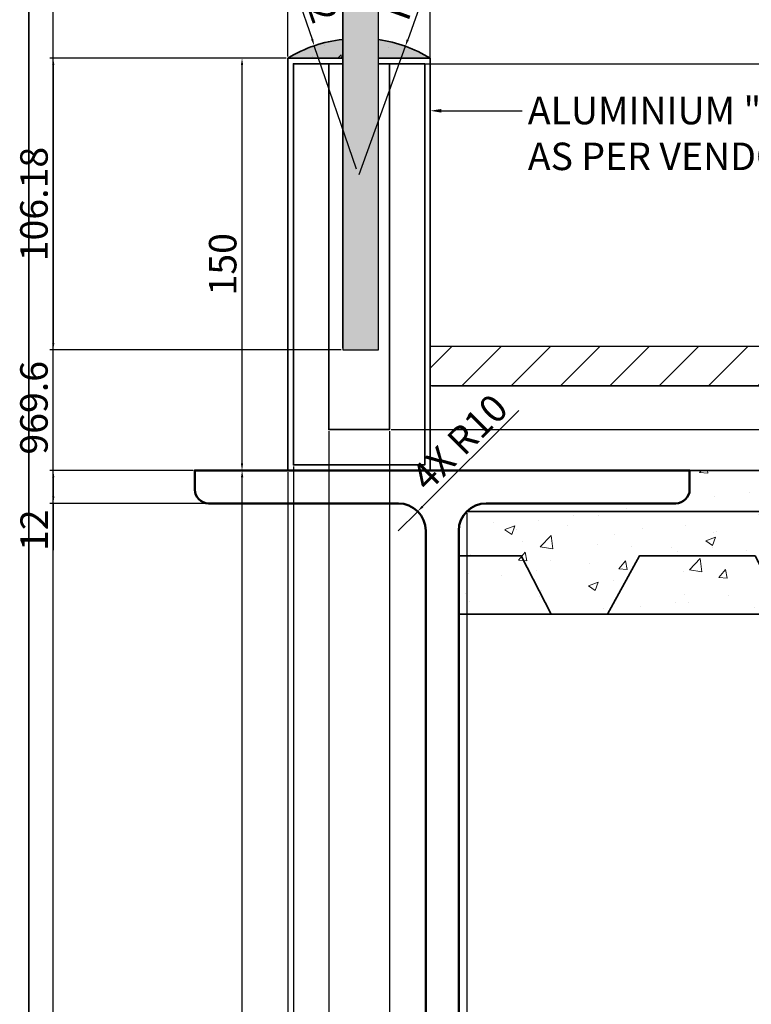
# Model space of a CAD drawing. Units: millimetres. Extents: x 1791 to 2420, y 1225 to 2361.
# Tile 2 of 4: x 1791 to 2057, y 1583 to 1941. Entities that reach past the tile are written whole.
import ezdxf
from ezdxf import colors
from ezdxf.entities.mleader import LeaderData, LeaderLine
from ezdxf.math import Vec2, Vec3

# ---------------------------------------------------------------- set-up
doc = ezdxf.new("R2010")
doc.units = ezdxf.units.MM
for name, color, linetype, lineweight in [('A-ANNO-DIMS', 2, 'Continuous', 18), ('A-ANNO-TEXT', 7, 'Continuous', 18), ('A-ANNO-TTLB', 7, 'Continuous', 35), ('A-DETL-PATT', 8, 'Continuous', 13), ('A-FLOR', 30, 'Continuous', 25), ('A-GLAZ', 5, 'Continuous', 25), ('A-RAIL', 4, 'Continuous', 35), ('S-BEAM', 1, 'Continuous', 50), ('S-DECK', 3, 'Continuous', 35)]:
    doc.layers.add(name, color=color, linetype=linetype, lineweight=lineweight)
doc.styles.get("Standard").update_dxf_attribs({"font": 'arial.ttf'})
doc.dimstyles.new('ISO-25', dxfattribs={"dimtxt": 10, "dimasz": 2.5, "dimexe": 1.25, "dimexo": 0.625, "dimtad": 1, "dimdec": 1, "dimtxsty": 'Standard', "dimcen": 2.5, "dimadec": 0, "dimazin": 0, "dimtfac": 1, "dimtdec": 1, "dimtmove": 0, "dimatfit": 3, "dimfxl": 1, "dimarcsym": 0})

# ---------------------------------------------------------------- blocks, each defined once
blk = doc.blocks.new('*D3')
at = {"layer": 'A-ANNO-DIMS', "color": 0, "lineweight": -2, "transparency": 16777216}
for p, q in [((1860.7, 1777.42), (1873.17, 1777.42)), ((1871.92, 1317.92), (1871.92, 1774.92)), ((1860.7, 1315.42), (1873.17, 1315.42))]:
    blk.add_line(p, q, dxfattribs=at)
at = {"layer": 'A-ANNO-DIMS', "color": 0, "transparency": 16777216}
for points in [[(1871.5, 1774.92), (1872.34, 1774.92), (1871.92, 1777.42)], [(1871.5, 1317.92), (1872.34, 1317.92), (1871.92, 1315.42)]]:
    blk.add_solid(points, dxfattribs=at)
at = {"layer": 'Defpoints', "color": 0, "transparency": 16777216}
for p in [(1860.08, 1777.42), (1871.92, 1777.42), (1860.08, 1315.42)]:
    blk.add_point(p, dxfattribs=at)
at = {"layer": 'A-ANNO-DIMS', "color": 0, "transparency": 16777216, "insert": (1866.19, 1546.42), "char_height": 10, "attachment_point": 5, "rotation": 90}
blk.add_mtext('462', dxfattribs=at)
blk = doc.blocks.new('*D4')
at = {"layer": 'A-ANNO-DIMS', "color": 0, "lineweight": -2, "transparency": 16777216}
for p, q in [((1887.99, 1927.42), (1870.65, 1927.42)), ((1871.9, 1779.92), (1871.9, 1924.92)), ((1887.99, 1777.42), (1870.65, 1777.42))]:
    blk.add_line(p, q, dxfattribs=at)
at = {"layer": 'A-ANNO-DIMS', "color": 0, "transparency": 16777216}
for points in [[(1871.48, 1924.92), (1872.31, 1924.92), (1871.9, 1927.42)], [(1871.48, 1779.92), (1872.31, 1779.92), (1871.9, 1777.42)]]:
    blk.add_solid(points, dxfattribs=at)
at = {"layer": 'Defpoints', "color": 0, "transparency": 16777216}
for p in [(1871.9, 1927.42), (1888.61, 1927.42), (1888.61, 1777.42)]:
    blk.add_point(p, dxfattribs=at)
at = {"layer": 'A-ANNO-DIMS', "color": 0, "transparency": 16777216, "insert": (1866.16, 1852.42), "char_height": 10, "attachment_point": 5, "rotation": 90}
blk.add_mtext('150', dxfattribs=at)
blk = doc.blocks.new('*D11')
at = {"layer": 'A-ANNO-DIMS', "color": 0, "lineweight": -2, "transparency": 16777216}
for p, q in [((1894.37, 2284.98), (1801.98, 2284.98)), ((1803.23, 1317.92), (1803.23, 2282.48)), ((1854.1, 1315.42), (1801.98, 1315.42))]:
    blk.add_line(p, q, dxfattribs=at)
at = {"layer": 'A-ANNO-DIMS', "color": 0, "transparency": 16777216}
for points in [[(1802.81, 2282.48), (1803.64, 2282.48), (1803.23, 2284.98)], [(1802.81, 1317.92), (1803.64, 1317.92), (1803.23, 1315.42)]]:
    blk.add_solid(points, dxfattribs=at)
at = {"layer": 'Defpoints', "color": 0, "transparency": 16777216}
for p in [(1803.23, 2284.98), (1895, 2284.98), (1854.73, 1315.42)]:
    blk.add_point(p, dxfattribs=at)
at = {"layer": 'A-ANNO-DIMS', "color": 0, "transparency": 16777216, "insert": (1797.5, 1800.2), "char_height": 10, "attachment_point": 5, "rotation": 90}
blk.add_mtext('969.6', dxfattribs=at)
blk = doc.blocks.new('*D12')
at = {"layer": 'A-ANNO-DIMS', "color": 0, "lineweight": -2, "transparency": 16777216}
for p, q in [((1908.56, 1821.87), (1908.56, 2350.12)), ((1911.06, 2348.87), (1919.06, 2348.87)), ((1921.56, 1821.87), (1921.56, 2350.12)), ((1921.56, 2348.87), (1938.7, 2348.87))]:
    blk.add_line(p, q, dxfattribs=at)
at = {"layer": 'A-ANNO-DIMS', "color": 0, "transparency": 16777216}
for points in [[(1911.06, 2349.29), (1911.06, 2348.45), (1908.56, 2348.87)], [(1919.06, 2349.29), (1919.06, 2348.45), (1921.56, 2348.87)]]:
    blk.add_solid(points, dxfattribs=at)
at = {"layer": 'Defpoints', "color": 0, "transparency": 16777216}
for p in [(1921.56, 2348.87), (1908.56, 1821.24), (1921.56, 1821.24)]:
    blk.add_point(p, dxfattribs=at)
at = {"layer": 'A-ANNO-DIMS', "color": 0, "transparency": 16777216, "insert": (1931.38, 2354.6), "char_height": 10, "attachment_point": 5}
blk.add_mtext('13', dxfattribs=at)
blk = doc.blocks.new('*D13')
at = {"layer": 'A-ANNO-DIMS', "color": 0, "lineweight": -2, "transparency": 16777216}
for p, q in [((1907.94, 2258.52), (1801.98, 2258.52)), ((1803.23, 1823.74), (1803.23, 2256.02)), ((1907.94, 1821.24), (1801.98, 1821.24))]:
    blk.add_line(p, q, dxfattribs=at)
at = {"layer": 'A-ANNO-DIMS', "color": 0, "transparency": 16777216}
for points in [[(1802.81, 2256.02), (1803.64, 2256.02), (1803.23, 2258.52)], [(1802.81, 1823.74), (1803.64, 1823.74), (1803.23, 1821.24)]]:
    blk.add_solid(points, dxfattribs=at)
at = {"layer": 'Defpoints', "color": 0, "transparency": 16777216}
for p in [(1803.23, 2258.52), (1908.56, 2258.52), (1908.56, 1821.24)]:
    blk.add_point(p, dxfattribs=at)
at = {"layer": 'A-ANNO-DIMS', "color": 0, "transparency": 16777216, "insert": (1797.49, 2039.88), "char_height": 10, "attachment_point": 5, "rotation": 90}
blk.add_mtext('437.3', dxfattribs=at)
blk = doc.blocks.new('*D14')
at = {"layer": 'A-ANNO-DIMS', "color": 0, "lineweight": -2, "transparency": 16777216}
for p, q in [((1887.99, 1927.42), (1801.98, 1927.42)), ((1803.23, 1924.92), (1803.23, 1823.74)), ((1907.94, 1821.24), (1801.98, 1821.24))]:
    blk.add_line(p, q, dxfattribs=at)
at = {"layer": 'A-ANNO-DIMS', "color": 0, "transparency": 16777216}
for points in [[(1802.81, 1924.92), (1803.64, 1924.92), (1803.23, 1927.42)], [(1802.81, 1823.74), (1803.64, 1823.74), (1803.23, 1821.24)]]:
    blk.add_solid(points, dxfattribs=at)
at = {"layer": 'Defpoints', "color": 0, "transparency": 16777216}
for p in [(1888.61, 1927.42), (1803.23, 1821.24), (1908.56, 1821.24)]:
    blk.add_point(p, dxfattribs=at)
at = {"layer": 'A-ANNO-DIMS', "color": 0, "transparency": 16777216, "insert": (1797.5, 1874.33), "char_height": 10, "attachment_point": 5, "rotation": 90}
blk.add_mtext('106.18', dxfattribs=at)
blk = doc.blocks.new('*D15')
at = {"layer": 'A-ANNO-DIMS', "color": 0, "lineweight": -2, "transparency": 16777216}
for p, q in [((1888.61, 1928.05), (1888.61, 2350.12)), ((1891.11, 2348.87), (1937.88, 2348.87)), ((1940.38, 1928.05), (1940.38, 2350.12))]:
    blk.add_line(p, q, dxfattribs=at)
at = {"layer": 'A-ANNO-DIMS', "color": 0, "transparency": 16777216}
for points in [[(1891.11, 2349.29), (1891.11, 2348.45), (1888.61, 2348.87)], [(1937.88, 2349.29), (1937.88, 2348.45), (1940.38, 2348.87)]]:
    blk.add_solid(points, dxfattribs=at)
at = {"layer": 'Defpoints', "color": 0, "transparency": 16777216}
for p in [(1940.38, 2348.87), (1888.61, 1927.42), (1940.38, 1927.42)]:
    blk.add_point(p, dxfattribs=at)
at = {"layer": 'A-ANNO-DIMS', "color": 0, "transparency": 16777216, "insert": (1914.5, 2354.6), "char_height": 10, "attachment_point": 5}
blk.add_mtext('51.76', dxfattribs=at)
blk = doc.blocks.new('*D16')
at = {"layer": 'A-ANNO-DIMS', "color": 0, "lineweight": -2, "transparency": 16777216}
for p, q in [((1890.61, 1778.8), (1890.61, 1262.67)), ((1888.61, 1776.8), (1888.61, 1262.67)), ((1886.11, 1263.92), (1883.61, 1263.92)), ((1888.61, 1263.92), (1890.61, 1263.92)), ((1893.11, 1263.92), (1903.49, 1263.92))]:
    blk.add_line(p, q, dxfattribs=at)
at = {"layer": 'A-ANNO-DIMS', "color": 0, "transparency": 16777216}
for points in [[(1886.11, 1264.34), (1886.11, 1263.5), (1888.61, 1263.92)], [(1893.11, 1264.34), (1893.11, 1263.5), (1890.61, 1263.92)]]:
    blk.add_solid(points, dxfattribs=at)
at = {"layer": 'Defpoints', "color": 0, "transparency": 16777216}
for p in [(1888.61, 1777.42), (1890.61, 1779.42), (1890.61, 1263.92)]:
    blk.add_point(p, dxfattribs=at)
at = {"layer": 'A-ANNO-DIMS', "color": 0, "transparency": 16777216, "insert": (1899.55, 1269.57), "char_height": 10, "attachment_point": 5}
blk.add_mtext('2', dxfattribs=at)
blk = doc.blocks.new('*D17')
at = {"layer": 'A-ANNO-DIMS', "color": 0, "lineweight": -2, "transparency": 16777216}
for p, q in [((1903.46, 1791.65), (1903.46, 1262.67)), ((1925.53, 1791.65), (1925.53, 1262.67)), ((1905.96, 1263.92), (1923.03, 1263.92)), ((1925.53, 1263.92), (1970.92, 1263.92))]:
    blk.add_line(p, q, dxfattribs=at)
at = {"layer": 'A-ANNO-DIMS', "color": 0, "transparency": 16777216}
for points in [[(1905.96, 1264.34), (1905.96, 1263.5), (1903.46, 1263.92)], [(1923.03, 1264.34), (1923.03, 1263.5), (1925.53, 1263.92)]]:
    blk.add_solid(points, dxfattribs=at)
at = {"layer": 'Defpoints', "color": 0, "transparency": 16777216}
for p in [(1903.46, 1792.27), (1925.53, 1792.27), (1925.53, 1263.92)]:
    blk.add_point(p, dxfattribs=at)
at = {"layer": 'A-ANNO-DIMS', "color": 0, "transparency": 16777216, "insert": (1949.47, 1269.65), "char_height": 10, "attachment_point": 5}
blk.add_mtext('22.064', dxfattribs=at)
blk = doc.blocks.new('*D18')
at = {"layer": 'A-ANNO-DIMS', "color": 0, "lineweight": -2, "transparency": 16777216}
for p, q in [((1926.15, 1925.42), (2419.97, 1925.42)), ((2418.72, 1922.92), (2418.72, 1794.77)), ((1926.15, 1792.27), (2419.97, 1792.27))]:
    blk.add_line(p, q, dxfattribs=at)
at = {"layer": 'A-ANNO-DIMS', "color": 0, "transparency": 16777216}
for points in [[(2418.3, 1922.92), (2419.13, 1922.92), (2418.72, 1925.42)], [(2418.3, 1794.77), (2419.13, 1794.77), (2418.72, 1792.27)]]:
    blk.add_solid(points, dxfattribs=at)
at = {"layer": 'Defpoints', "color": 0, "transparency": 16777216}
for p in [(1925.53, 1925.42), (1925.53, 1792.27), (2418.72, 1792.27)]:
    blk.add_point(p, dxfattribs=at)
at = {"layer": 'A-ANNO-DIMS', "color": 0, "transparency": 16777216, "insert": (2412.98, 1858.85), "char_height": 10, "attachment_point": 5, "rotation": 90}
blk.add_mtext('133.15', dxfattribs=at)
blk = doc.blocks.new('*D19')
at = {"layer": 'A-ANNO-DIMS', "color": 0, "lineweight": -2, "transparency": 16777216}
for p, q in [((2418.72, 1822.58), (2418.72, 1866.9)), ((1941, 1822.58), (2419.97, 1822.58)), ((2418.72, 1810.65), (2418.72, 1820.08)), ((1941, 1808.15), (2419.97, 1808.15))]:
    blk.add_line(p, q, dxfattribs=at)
at = {"layer": 'A-ANNO-DIMS', "color": 0, "transparency": 16777216}
for points in [[(2418.3, 1820.08), (2419.13, 1820.08), (2418.72, 1822.58)], [(2418.3, 1810.65), (2419.13, 1810.65), (2418.72, 1808.15)]]:
    blk.add_solid(points, dxfattribs=at)
at = {"layer": 'Defpoints', "color": 0, "transparency": 16777216}
for p in [(1940.38, 1822.58), (2418.72, 1822.58), (1940.38, 1808.15)]:
    blk.add_point(p, dxfattribs=at)
at = {"layer": 'A-ANNO-DIMS', "color": 0, "transparency": 16777216, "insert": (2412.98, 1845.99), "char_height": 10, "attachment_point": 5, "rotation": 90}
blk.add_mtext('14.423', dxfattribs=at)
blk = doc.blocks.new('*D21')
at = {"layer": 'A-ANNO-DIMS', "color": 0, "lineweight": -2, "transparency": 16777216}
for p, q in [((1854.1, 1777.42), (1801.98, 1777.42)), ((1803.23, 1774.92), (1803.23, 1767.92)), ((1859.1, 1765.42), (1801.98, 1765.42)), ((1803.23, 1765.42), (1803.23, 1748.39))]:
    blk.add_line(p, q, dxfattribs=at)
at = {"layer": 'A-ANNO-DIMS', "color": 0, "transparency": 16777216}
for points in [[(1802.81, 1774.92), (1803.64, 1774.92), (1803.23, 1777.42)], [(1802.81, 1767.92), (1803.64, 1767.92), (1803.23, 1765.42)]]:
    blk.add_solid(points, dxfattribs=at)
at = {"layer": 'Defpoints', "color": 0, "transparency": 16777216}
for p in [(1854.73, 1777.42), (1803.23, 1765.42), (1859.73, 1765.42)]:
    blk.add_point(p, dxfattribs=at)
at = {"layer": 'A-ANNO-DIMS', "color": 0, "transparency": 16777216, "insert": (1797.58, 1755.66), "char_height": 10, "attachment_point": 5, "rotation": 90}
blk.add_mtext('12', dxfattribs=at)
blk = doc.blocks.new('*D27')
at = {"layer": 'A-ANNO-DIMS', "color": 0, "lineweight": -2, "transparency": 16777216}
for p, q in [((1940.38, 1808.78), (1940.38, 2350.12)), ((1942.88, 2348.87), (2184.03, 2348.87)), ((2186.53, 1808.78), (2186.53, 2350.12))]:
    blk.add_line(p, q, dxfattribs=at)
at = {"layer": 'A-ANNO-DIMS', "color": 0, "transparency": 16777216}
for points in [[(1942.88, 2349.29), (1942.88, 2348.45), (1940.38, 2348.87)], [(2184.03, 2349.29), (2184.03, 2348.45), (2186.53, 2348.87)]]:
    blk.add_solid(points, dxfattribs=at)
at = {"layer": 'Defpoints', "color": 0, "transparency": 16777216}
for p in [(2186.53, 2348.87), (1940.38, 1808.15), (2186.53, 1808.15)]:
    blk.add_point(p, dxfattribs=at)
at = {"layer": 'A-ANNO-DIMS', "color": 0, "transparency": 16777216, "insert": (2063.45, 2354.6), "char_height": 10, "attachment_point": 5}
blk.add_mtext('246.15', dxfattribs=at)
blk = doc.blocks.new('*D32')
at = {"layer": 'A-ANNO-DIMS', "color": 0, "lineweight": -2, "transparency": 16777216}
for p, q in [((2077.9, 1766.79), (2077.9, 1262.67)), ((1953.66, 1761.87), (1953.66, 1262.67)), ((1956.16, 1263.92), (2075.4, 1263.92))]:
    blk.add_line(p, q, dxfattribs=at)
at = {"layer": 'A-ANNO-DIMS', "color": 0, "transparency": 16777216}
for points in [[(1956.16, 1264.34), (1956.16, 1263.5), (1953.66, 1263.92)], [(2075.4, 1264.34), (2075.4, 1263.5), (2077.9, 1263.92)]]:
    blk.add_solid(points, dxfattribs=at)
at = {"layer": 'Defpoints', "color": 0, "transparency": 16777216}
for p in [(2077.9, 1767.42), (1953.66, 1762.49), (2077.9, 1263.92)]:
    blk.add_point(p, dxfattribs=at)
at = {"layer": 'A-ANNO-DIMS', "color": 0, "transparency": 16777216, "insert": (2015.78, 1269.57), "char_height": 10, "attachment_point": 5}
blk.add_mtext('124.24', dxfattribs=at)
blk = doc.blocks.new('*D38')
at = {"layer": 'A-ANNO-DIMS', "color": 0, "lineweight": -2, "transparency": 16777216}
for p, q in [((1972.57, 1799.26), (1937.57, 1764.26)), ((1928.73, 1755.42), (1935.8, 1762.49))]:
    blk.add_line(p, q, dxfattribs=at)
at = {"layer": 'A-ANNO-DIMS', "color": 0, "transparency": 16777216}
blk.add_solid([(1937.27, 1764.55), (1937.86, 1763.97), (1935.8, 1762.49)], dxfattribs=at)
at = {"layer": 'Defpoints', "color": 0, "transparency": 16777216}
for p in [(1935.8, 1762.49), (1928.73, 1755.42)]:
    blk.add_point(p, dxfattribs=at)
at = {"layer": 'A-ANNO-DIMS', "color": 0, "transparency": 16777216, "insert": (1951.9, 1786.7), "char_height": 10, "attachment_point": 5, "rotation": 45.0016}
blk.add_mtext('4X R10', dxfattribs=at)
blk = doc.blocks.new('*D40')
at = {"layer": 'A-ANNO-DIMS', "color": 0, "lineweight": -2, "transparency": 16777216}
for p, q in [((1948.97, 1980.8), (1932.16, 1934.12)), ((1914.5, 1885.05), (1931.31, 1931.76))]:
    blk.add_line(p, q, dxfattribs=at)
at = {"layer": 'A-ANNO-DIMS', "color": 0, "transparency": 16777216}
blk.add_solid([(1931.77, 1934.26), (1932.55, 1933.98), (1931.31, 1931.76)], dxfattribs=at)
at = {"layer": 'Defpoints', "color": 0, "transparency": 16777216}
for p in [(1931.31, 1931.76), (1914.5, 1885.05)]:
    blk.add_point(p, dxfattribs=at)
at = {"layer": 'A-ANNO-DIMS', "color": 0, "transparency": 16777216, "insert": (1936.01, 1961.74), "char_height": 10, "attachment_point": 5, "rotation": 70.2009}
blk.add_mtext('R49.65', dxfattribs=at)
blk = doc.blocks.new('*D41')
at = {"layer": 'A-ANNO-DIMS', "color": 0, "lineweight": -2, "transparency": 16777216}
for p, q in [((1881.8, 1979.97), (1897.4, 1934.31)), ((1913.57, 1886.98), (1898.2, 1931.95))]:
    blk.add_line(p, q, dxfattribs=at)
at = {"layer": 'A-ANNO-DIMS', "color": 0, "transparency": 16777216}
blk.add_solid([(1897.79, 1934.45), (1897, 1934.18), (1898.2, 1931.95)], dxfattribs=at)
at = {"layer": 'Defpoints', "color": 0, "transparency": 16777216}
for p in [(1898.2, 1931.95), (1913.57, 1886.98)]:
    blk.add_point(p, dxfattribs=at)
at = {"layer": 'A-ANNO-DIMS', "color": 0, "transparency": 16777216, "insert": (1894.41, 1960.78), "char_height": 10, "attachment_point": 5, "rotation": 288.8663}
blk.add_mtext('R47.52', dxfattribs=at)

msp = doc.modelspace()

# ---------------------------------------------------------------- hatches: boundary and pattern name
at = {"layer": 'A-DETL-PATT'}
h = msp.add_hatch(color=256, dxfattribs=at)
h.dxf.hatch_style = 1
h.paths.add_polyline_path([(1921.5621, 2258.5157), (1908.5621, 2258.5157), (1908.5621, 1821.2446), (1921.5621, 1821.2446)])
h = msp.add_hatch(dxfattribs=at)
h.set_pattern_fill('AR-CONC', color=256, scale=0.1)
h.paths.add_polyline_path([(1908.5621, 1934.2375, 0.11230819), (1888.6133, 1927.4206), (1908.5621, 1927.4206)])
h.paths.add_polyline_path([(1921.5621, 1934.1943), (1921.5621, 1927.4206), (1940.378, 1927.4206, 0.10172817)])
h = msp.add_hatch(dxfattribs=at)
h.set_pattern_fill('AR-SAND', color=256, scale=0.01)
h.paths.add_polyline_path([(1908.5621, 1934.2375, 0.11230819), (1888.6133, 1927.4206), (1908.5621, 1927.4206)])
h.paths.add_polyline_path([(1921.5621, 1934.1943), (1921.5621, 1927.4206), (1940.378, 1927.4206, 0.10172817)])
h = msp.add_hatch(dxfattribs=at)
h.set_pattern_fill('ANSI31', color=256, scale=4)
h.paths.add_polyline_path([(2186.5283, 1822.576), (2063.4532, 1822.576), (1940.378, 1822.576), (1940.378, 1808.1531), (2186.5283, 1808.1531)])
h.paths.add_polyline_path([(2367.2176, 1836.999), (2063.4532, 1836.999), (2063.4532, 1822.576), (2367.2176, 1822.576)])
h = msp.add_hatch(dxfattribs=at)
h.set_pattern_fill('AR-CONC', color=256, scale=0.2)
h.paths.add_polyline_path([(2058.5452, 1746.3347), (2035.8237, 1746.3347), (2030.2178, 1746.3347), (2016.5047, 1746.3347), (2004.8892, 1725.0563), (2069.4909, 1725.0563)], flags=17)
h.paths.add_polyline_path([(2166.1796, 1767.4162, -0.41421356), (2161.2551, 1762.4917), (2167.6174, 1762.4917), (2243.8358, 1762.4917, -0.41421356), (2238.9113, 1767.4162, -1), (2248.7603, 1767.4162, -0.41421356), (2243.8358, 1762.4917), (2250.3259, 1762.4917), (2325.7548, 1762.4917, -0.41421356), (2320.8303, 1767.4162, -1), (2330.6793, 1767.4162, -0.41421356), (2325.7548, 1762.4917), (2331.0978, 1762.4917), (2367.2176, 1762.4917), (2367.2176, 1777.4206), (2034.727, 1777.4206), (2034.727, 1770.4206, -0.41421356), (2029.727, 1765.4206), (1960.727, 1765.4206, 0.19891237), (1953.6559, 1762.4917), (2077.8995, 1762.4917, -0.41421356), (2072.975, 1767.4162, -1), (2082.824, 1767.4162, -0.41421356), (2077.8995, 1762.4917), (2083.2584, 1762.4917), (2161.2551, 1762.4917, -0.41421356), (2156.3306, 1767.4162, -1)])
h.paths.add_polyline_path([(2016.5047, 1746.3347), (2030.2178, 1746.3347), (2035.8237, 1746.3347), (2058.5452, 1746.3347), (2069.4909, 1725.0563), (2073.0274, 1725.0563, -0.30569965), (2076.7379, 1729.1256), (2076.7379, 1759.0444), (2072.3578, 1759.0444), (2072.3578, 1762.4917), (1953.6559, 1762.4917, 0.19891237), (1950.727, 1755.4206), (1950.727, 1746.3347), (1973.4485, 1746.3347), (1984.3943, 1725.0563), (2004.8892, 1725.0563)])
h.paths.add_polyline_path([(1973.4485, 1746.3347), (1950.727, 1746.3347), (1950.727, 1725.0563), (1984.3943, 1725.0563)], flags=17)
h.paths.add_polyline_path([(2140.839, 1746.3347), (2118.1174, 1746.3347), (2115.3145, 1746.3347), (2101.6014, 1746.3347), (2089.9858, 1725.0563), (2151.7847, 1725.0563)], flags=17)
h.paths.add_polyline_path([(2161.0969, 1759.0444), (2156.7168, 1759.0444), (2156.7168, 1762.4917), (2083.2584, 1762.4917), (2083.2584, 1758.968), (2079.2222, 1758.968), (2079.2222, 1729.0836, -0.29648266), (2082.7716, 1725.0563), (2089.9858, 1725.0563), (2101.6014, 1746.3347), (2115.3145, 1746.3347), (2120.9204, 1746.3347), (2140.839, 1746.3347), (2151.7847, 1725.0563), (2157.0332, 1725.0563, -0.35098402), (2161.0969, 1729.6797)])
h.paths.add_polyline_path([(2243.8053, 1759.0444), (2239.4253, 1759.0444), (2239.4253, 1762.4917), (2167.6174, 1762.4917), (2167.6174, 1758.968), (2163.5811, 1758.968), (2163.5811, 1729.4775, -0.30598924), (2166.8718, 1725.0563), (2172.2796, 1725.0563), (2183.8952, 1746.3347), (2197.6083, 1746.3347), (2203.2141, 1746.3347), (2223.1327, 1746.3347), (2234.0785, 1725.0563), (2240.3204, 1725.0563, -0.34708966), (2243.8053, 1730.0651)])
h.paths.add_polyline_path([(2223.1327, 1746.3347), (2200.4112, 1746.3347), (2197.6083, 1746.3347), (2183.8952, 1746.3347), (2172.2796, 1725.0563), (2234.0785, 1725.0563)], flags=17)
h.paths.add_polyline_path([(2324.5773, 1759.0444), (2320.1972, 1759.0444), (2320.1972, 1762.4917), (2250.3259, 1762.4917), (2250.3259, 1758.968), (2246.2896, 1758.968), (2246.2896, 1730.1635, -0.36941305), (2250.1515, 1725.0563), (2254.5734, 1725.0563), (2266.1889, 1746.3347), (2279.902, 1746.3347), (2285.5079, 1746.3347), (2305.4265, 1746.3347), (2316.3722, 1725.0563), (2320.8471, 1725.0563, -0.36687812), (2324.5773, 1730.2193)])
h.paths.add_polyline_path([(2305.4265, 1746.3347), (2282.705, 1746.3347), (2279.902, 1746.3347), (2266.1889, 1746.3347), (2254.5734, 1725.0563), (2316.3722, 1725.0563)], flags=17)
h.paths.add_polyline_path([(2367.2176, 1762.4917), (2331.0978, 1762.4917), (2331.0978, 1758.968), (2327.0615, 1758.968), (2327.0615, 1730.1866, -0.3594453), (2330.6665, 1725.0563), (2336.8671, 1725.0563), (2348.4827, 1746.3347), (2362.1958, 1746.3347), (2367.2176, 1746.3347)])
h.paths.add_polyline_path([(2367.2176, 1746.3347), (2362.1958, 1746.3347), (2348.4827, 1746.3347), (2336.8671, 1725.0563), (2367.2176, 1725.0563)], flags=17)

# ---------------------------------------------------------------- linework, layer by layer
at = {"layer": 'A-ANNO-TTLB'}
msp.add_line((1794.3467, 1287.0028), (1794.3467, 2307.8191), dxfattribs=at)
at = {"layer": 'A-FLOR'}
msp.add_lwpolyline([(1940.378, 1822.576), (2186.5283, 1822.576), (2186.5283, 1808.1531), (1940.378, 1808.1531)], close=True, dxfattribs=at)
at = {"layer": 'A-GLAZ'}
msp.add_lwpolyline([(1908.5621, 1821.2446), (1921.5621, 1821.2446), (1921.5621, 2258.5157), (1908.5621, 2258.5157)], close=True, dxfattribs=at)
at = {"layer": 'A-RAIL'}
for points in [[(1908.5621, 1927.4206), (1888.6133, 1927.4206), (1888.6133, 1777.4206), (1940.378, 1777.4206), (1940.378, 1927.4206), (1921.5621, 1927.4206)], [(1907.7361, 1925.4206), (1890.6133, 1925.4206), (1890.6133, 1779.4206), (1938.378, 1779.4206), (1938.378, 1925.4206), (1921.5621, 1925.4206)], [(1908.5621, 1925.4206), (1903.4637, 1925.4206), (1903.4637, 1792.271), (1925.5277, 1792.271), (1925.5277, 1925.4206), (1921.5621, 1925.4206)]]:
    msp.add_lwpolyline(points, dxfattribs=at)
for centre, radius, start, end in [((1913.5708, 1886.9827), 47.5194, 96.050403, 121.682138), ((1914.4957, 1885.0453), 49.6544, 58.583851, 81.818303)]:
    msp.add_arc(centre, radius, start, end, dxfattribs=at)
at = {"layer": 'S-BEAM'}
msp.add_lwpolyline([(1938.727, 1755.4206, 0.41421356), (1928.727, 1765.4206), (1859.727, 1765.4206, -0.41421356), (1854.727, 1770.4206), (1854.727, 1777.4206), (2034.727, 1777.4206), (2034.727, 1770.4206, -0.41421356), (2029.727, 1765.4206), (1960.727, 1765.4206, 0.41421356), (1950.727, 1755.4206), (1950.727, 1337.4206, 0.41421356), (1960.727, 1327.4206), (2029.727, 1327.4206, -0.41421356), (2034.727, 1322.4206), (2034.727, 1315.4206), (1854.727, 1315.4206), (1854.727, 1322.4206, -0.41421356), (1859.727, 1327.4206), (1928.727, 1327.4206, 0.41421356), (1938.727, 1337.4206), (1938.727, 1755.4206)], format="xyb", dxfattribs=at)
at = {"layer": 'S-DECK'}
for p, q in [((1854.727, 1777.4206), (2367.2176, 1777.4206)), ((1953.6559, 1762.4917), (2367.2176, 1762.4917)), ((1950.727, 1725.0563), (2367.2176, 1725.0563))]:
    msp.add_line(p, q, dxfattribs=at)
for points in [[(1950.727, 1746.3347), (1973.4485, 1746.3347), (1984.3943, 1725.0563), (2004.8892, 1725.0563), (2016.5047, 1746.3347), (2030.2178, 1746.3347), (2035.8237, 1746.3347)], [(2035.8237, 1746.3347), (2058.5452, 1746.3347), (2069.4909, 1725.0563), (2089.9858, 1725.0563), (2101.6014, 1746.3347), (2115.3145, 1746.3347), (2120.9204, 1746.3347)]]:
    msp.add_lwpolyline(points, dxfattribs=at)

# ---------------------------------------------------------------- dimensions: what is measured, and where the dimension line sits
at = {"layer": 'A-ANNO-DIMS'}
for base, p1, p2, override, picture, middle in [((1940.378, 2348.8684), (1888.6133, 1927.4206), (1940.378, 1927.4206), {"dimdec": 2, "dimlfac": 1, "dimrnd": 0, "dimzin": 0, "dimdsep": 46, "dimlunit": 2}, '*D15', (1914.4957, 2354.5991)), ((1921.5621, 2348.8684), (1908.5621, 1821.2446), (1921.5621, 1821.2446), {"dimdec": 0, "dimlfac": 1, "dimrnd": 0, "dimzin": 0, "dimdsep": 46, "dimlunit": 2}, '*D12', (1931.3788, 2354.6025)), ((2186.5283, 2348.8684), (1940.378, 1808.1531), (2186.5283, 1808.1531), {"dimdec": 2, "dimlfac": 1, "dimrnd": 0, "dimzin": 0, "dimdsep": 46, "dimlunit": 2}, '*D27', (2063.4532, 2354.5991)), ((1925.5277, 1263.9206), (1903.4637, 1792.271), (1925.5277, 1792.271), {"dimdec": 3, "dimlfac": 1, "dimrnd": 0, "dimzin": 0, "dimdsep": 46, "dimlunit": 2}, '*D17', (1949.4746, 1269.6513)), ((1890.6133, 1263.9206), (1888.6133, 1777.4206), (1890.6133, 1779.4206), {"dimdec": 0, "dimlfac": 1, "dimrnd": 0, "dimzin": 0, "dimdsep": 46, "dimlunit": 2}, '*D16', (1899.5501, 1269.566)), ((2077.8995, 1263.9206), (1953.6559, 1762.4917), (2077.8995, 1767.4162), {"dimdec": 2, "dimlfac": 1, "dimrnd": 0, "dimzin": 0, "dimdsep": 46, "dimlunit": 2}, '*D32', (2015.7777, 1269.566))]:
    dim = msp.add_linear_dim(base=base, p1=p1, p2=p2, dimstyle='ISO-25', override=override, dxfattribs=at)
    dim.commit()
    dim.dimension.update_dxf_attribs({"geometry": picture, "text_midpoint": middle})
for base, p1, p2, override, picture, middle in [((1803.227, 2284.9823), (1854.727, 1315.4206), (1894.9953, 2284.9823), {"dimdec": 1, "dimlfac": 1, "dimrnd": 0, "dimzin": 0, "dimdsep": 46, "dimlunit": 2}, '*D11', (1797.4963, 1800.2015)), ((1803.227, 2258.5157), (1908.5621, 1821.2446), (1908.5621, 2258.5157), {"dimdec": 1, "dimlfac": 1, "dimrnd": 0, "dimzin": 0, "dimdsep": 46, "dimlunit": 2}, '*D13', (1797.4929, 2039.8801)), ((1803.227, 1821.2446), (1888.6133, 1927.4206), (1908.5621, 1821.2446), {"dimdec": 2, "dimlfac": 1, "dimrnd": 0, "dimzin": 0, "dimdsep": 46, "dimlunit": 2}, '*D14', (1797.4963, 1874.3326)), ((2418.7176, 1792.271), (1925.5277, 1925.4206), (1925.5277, 1792.271), {"dimdec": 2, "dimlfac": 1, "dimrnd": 0, "dimzin": 0, "dimdsep": 46, "dimlunit": 2}, '*D18', (2412.9835, 1858.8458)), ((2418.7176, 1822.576), (1940.378, 1808.1531), (1940.378, 1822.576), {"dimdec": 3, "dimlfac": 1, "dimrnd": 0, "dimzin": 0, "dimdsep": 46, "dimlunit": 2}, '*D19', (2412.9835, 1845.9875)), ((1803.227, 1765.4206), (1854.727, 1777.4206), (1859.727, 1765.4206), {"dimdec": 0, "dimlfac": 1, "dimrnd": 0, "dimzin": 0, "dimdsep": 46, "dimlunit": 2}, '*D21', (1797.5815, 1755.6551))]:
    dim = msp.add_linear_dim(base=base, p1=p1, p2=p2, angle=90, dimstyle='ISO-25', override=override, dxfattribs=at)
    dim.commit()
    dim.dimension.update_dxf_attribs({"geometry": picture, "text_midpoint": middle})
for center, mpoint, picture, middle in [((1913.5708, 1886.9827), (1898.2049, 1931.9492), '*D41', (1888.9854, 1958.9291)), ((1914.4957, 1885.0453), (1931.3148, 1931.7644), '*D40', (1941.4063, 1959.7959))]:
    dim = msp.add_radius_dim(center=center, mpoint=mpoint, dimstyle='ISO-25', override={"dimdec": 2, "dimlfac": 1, "dimrnd": 0, "dimzin": 0, "dimdsep": 46, "dimlunit": 2}, dxfattribs=at)
    dim.commit()
    dim.dimension.update_dxf_attribs({"geometry": picture, "text_midpoint": middle, "dimtype": 164})
for p1, p2, distance, picture, middle in [((1888.6133, 1777.4206), (1888.6133, 1927.4206), 16.7182, '*D4', (1866.1644, 1852.4206)), ((1860.0795, 1315.4206), (1860.0795, 1777.4206), -11.8389, '*D3', (1866.1876, 1546.4206))]:
    dim = msp.add_aligned_dim(p1=p1, p2=p2, distance=distance, dimstyle='ISO-25', override={"dimclrd": 0, "dimclre": 0, "dimclrt": 0}, dxfattribs=at)
    dim.commit()
    dim.dimension.update_dxf_attribs({"geometry": picture, "text_midpoint": middle})
dim = msp.add_radius_dim(center=(1928.727, 1755.4206), mpoint=(1935.7979, 1762.4919), text='4X <>', dimstyle='ISO-25', override={"dimdec": 0, "dimlfac": 1, "dimrnd": 0, "dimzin": 0, "dimdsep": 46, "dimlunit": 2}, dxfattribs=at)
dim.commit()
dim.dimension.update_dxf_attribs({"geometry": '*D38', "text_midpoint": (1951.8976, 1786.6972)})

# ---------------------------------------------------------------- leaders
at = {"layer": 'A-ANNO-TEXT'}
ml = msp.add_multileader_mtext('Standard', dxfattribs=at)
ml.set_content('ALUMINIUM " U CHANNEL BASE SUPPORT\\PAS PER VENDOR DETAIL', color=256)
ml.set_leader_properties()
ml.build(insert=Vec2(0, 0))
ctx = ml.context
ctx.base_point, ctx.char_height, ctx.plane_origin = Vec3(1973.8617, 1908.272), 10, Vec3(1940.378, 1908.272)
notes = []
notes.append((ctx, [(0, (1, 1, 0), (1965.8617, 1908.272), (1, 0), 8, [(0, [(1940.378, 1908.272)], 0, [])])]))
ctx.mtext.insert, ctx.mtext.flow_direction = Vec3(1975.8617, 1913.3573), 5
for ctx, leaders in notes:
    for number, flags, end, landing, length, lines in leaders:
        leader = LeaderData()
        leader.index, (leader.has_last_leader_line, leader.has_dogleg_vector, leader.attachment_direction) = number, flags
        leader.last_leader_point, leader.dogleg_vector, leader.dogleg_length = Vec3(end), Vec3(landing), length
        for number, points, colour, breaks in lines:
            line = LeaderLine()
            line.index, line.vertices, line.color, line.breaks = number, Vec3.list(points), colors.encode_raw_color(colour), breaks
            leader.lines.append(line)
        ctx.leaders.append(leader)

doc.saveas('drawing.dxf')
